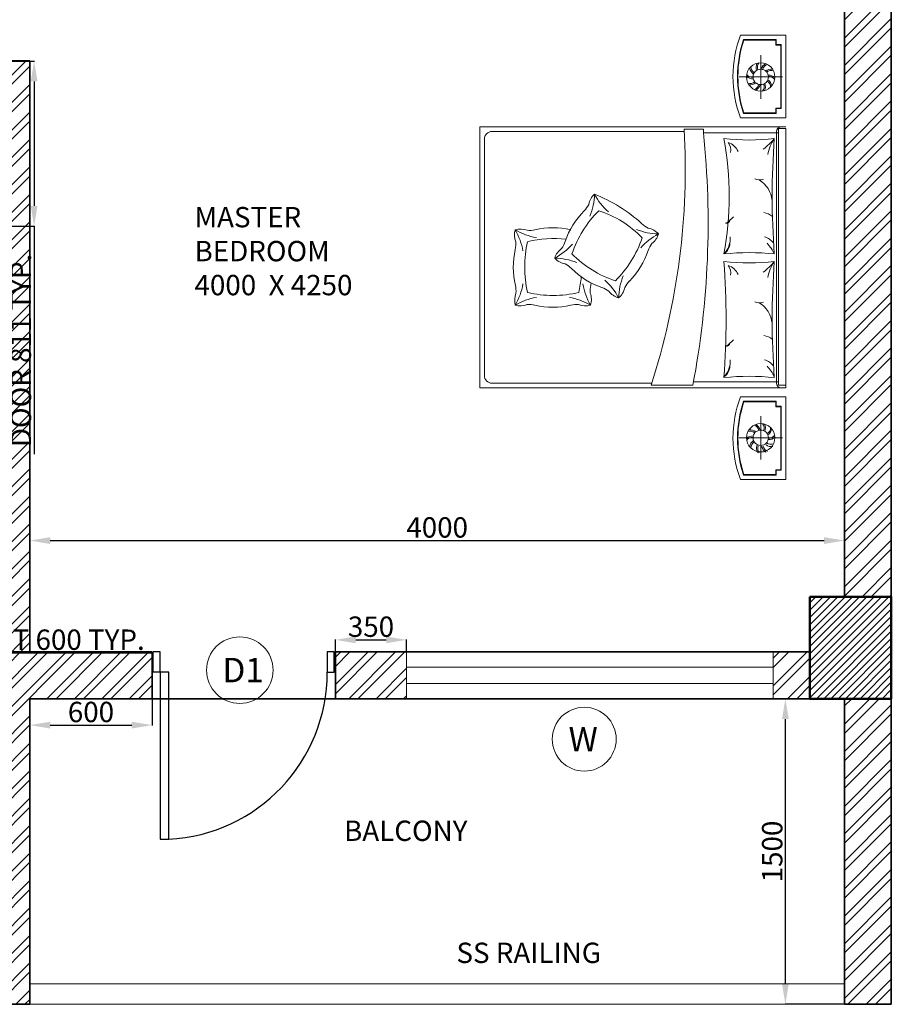
# Model space of a CAD drawing. Units: millimetres. Extents: x -3326 to 29338, y -16792 to 6002.
# Tile 16 of 21: x 25002 to 29282, y -12764 to -7931. Entities that reach past the tile are written whole.
import ezdxf

# ---------------------------------------------------------------- set-up
doc = ezdxf.new("R2010")
doc.units = ezdxf.units.MM
doc.header["$PDMODE"] = 35
doc.header["$PDSIZE"] = 5
for name, color, linetype, lineweight in [('A-ANNO-DIMS', 2, 'Continuous', 13), ('A-ANNO-SYMB', 7, 'Continuous', 18), ('A-AREA-IDEN', 7, 'Continuous', 18), ('A-COLS', 1, 'Continuous', 50), ('A-COLS-PATT', 251, 'Continuous', 13), ('A-DOOR', 3, 'Continuous', 25), ('A-FLOR-RAIL', 8, 'Continuous', 20), ('A-GLAZ', 4, 'Continuous', 18), ('A-WALL', 7, 'Continuous', 35), ('A-WALL-PATT', 252, 'Continuous', 13), ('furn', 28, 'Continuous', 18), ('txt', 7, 'Continuous', 18)]:
    doc.layers.add(name, color=color, linetype=linetype, lineweight=lineweight)
doc.styles.get("Standard").update_dxf_attribs({"font": 'arial.ttf'})
doc.dimstyles.new('ISO-25', dxfattribs={"dimtxt": 100, "dimasz": 100, "dimexe": 1.25, "dimexo": 0.625, "dimtad": 1, "dimtxsty": 'Standard', "dimcen": 2.5, "dimadec": 0, "dimazin": 0, "dimtfac": 1, "dimtmove": 0, "dimatfit": 3, "dimfxl": 1, "dimarcsym": 0})

# ---------------------------------------------------------------- blocks, each defined once
blk = doc.blocks.new('A$C0CE462CD')
for p, q in [((860, 100), (860, 0)), ((860, 0), (893.9, 0))]:
    blk.add_line(p, q)
for points in [[(860, 100), (860, 920), (818.4, 920), (818.4, 100)], [(0, 10), (6.1, 10), (6.1, 90), (0, 90)], [(893.9, 10), (900, 10), (900, 90), (893.9, 90)]]:
    blk.add_lwpolyline(points, close=True)
for points in [[(6.1, 0), (40, 0), (40, 100), (6.1, 100)], [(6.1, 100), (6.1, 0)], [(860, 100), (893.9, 100), (893.9, 0)]]:
    blk.add_lwpolyline(points)
blk.add_arc((859.1, 101.9), 819.1, 92.8508, 180.1309)
blk = doc.blocks.new('*D12')
at = {"layer": 'A-ANNO-DIMS', "color": 0, "lineweight": -2, "transparency": 16777216}
for p, q in [((29051.7, -11264), (28760.9, -11264)), ((28762.1, -12664), (28762.1, -11364)), ((29051.7, -12764), (28760.9, -12764))]:
    blk.add_line(p, q, dxfattribs=at)
at = {"layer": 'A-ANNO-DIMS', "color": 0, "transparency": 16777216}
for points in [[(28745.4, -11364), (28778.8, -11364), (28762.1, -11264)], [(28745.4, -12664), (28778.8, -12664), (28762.1, -12764)]]:
    blk.add_solid(points, dxfattribs=at)
at = {"layer": 'Defpoints', "color": 0, "transparency": 16777216}
for p in [(28762.1, -11264), (29052.3, -11264), (29052.3, -12764)]:
    blk.add_point(p, dxfattribs=at)
at = {"layer": 'A-ANNO-DIMS', "color": 0, "transparency": 16777216, "insert": (28710.4, -12014), "char_height": 100, "attachment_point": 5, "rotation": 90}
blk.add_mtext('1500', dxfattribs=at)
blk = doc.blocks.new('*D13')
at = {"layer": 'A-ANNO-DIMS', "color": 0, "lineweight": -2, "transparency": 16777216}
for p, q in [((25052.3, -11264.6), (25052.3, -11395)), ((25652.3, -11264.6), (25652.3, -11395)), ((25152.3, -11393.8), (25552.3, -11393.8))]:
    blk.add_line(p, q, dxfattribs=at)
at = {"layer": 'A-ANNO-DIMS', "color": 0, "transparency": 16777216}
for points in [[(25152.3, -11377.1), (25152.3, -11410.4), (25052.3, -11393.8)], [(25552.3, -11377.1), (25552.3, -11410.4), (25652.3, -11393.8)]]:
    blk.add_solid(points, dxfattribs=at)
at = {"layer": 'Defpoints', "color": 0, "transparency": 16777216}
for p in [(25052.3, -11264), (25652.3, -11264), (25652.3, -11393.8)]:
    blk.add_point(p, dxfattribs=at)
at = {"layer": 'A-ANNO-DIMS', "color": 0, "transparency": 16777216, "insert": (25352.3, -11342.1), "char_height": 100, "attachment_point": 5}
blk.add_mtext('600', dxfattribs=at)
blk = doc.blocks.new('*D14')
at = {"layer": 'A-ANNO-DIMS', "color": 0, "lineweight": -2, "transparency": 16777216}
for p, q in [((26552.3, -11033.3), (26552.3, -10973.9)), ((26652.3, -10975.2), (26802.3, -10975.2)), ((26902.3, -11033.3), (26902.3, -10973.9))]:
    blk.add_line(p, q, dxfattribs=at)
at = {"layer": 'A-ANNO-DIMS', "color": 0, "transparency": 16777216}
for points in [[(26652.3, -10958.5), (26652.3, -10991.9), (26552.3, -10975.2)], [(26802.3, -10958.5), (26802.3, -10991.9), (26902.3, -10975.2)]]:
    blk.add_solid(points, dxfattribs=at)
at = {"layer": 'Defpoints', "color": 0, "transparency": 16777216}
for p in [(26902.3, -10975.2), (26552.3, -11034), (26902.3, -11034)]:
    blk.add_point(p, dxfattribs=at)
at = {"layer": 'A-ANNO-DIMS', "color": 0, "transparency": 16777216, "insert": (26727.3, -10923.5), "char_height": 100, "attachment_point": 5}
blk.add_mtext('350', dxfattribs=at)
blk = doc.blocks.new('*D15')
at = {"layer": 'A-ANNO-DIMS', "color": 0, "lineweight": -2, "transparency": 16777216}
for p, q in [((29052.3, -10333.7), (29052.3, -10489.2)), ((25052.3, -10425.5), (25052.3, -10489.2)), ((25152.3, -10487.9), (28952.3, -10487.9))]:
    blk.add_line(p, q, dxfattribs=at)
at = {"layer": 'A-ANNO-DIMS', "color": 0, "transparency": 16777216}
for points in [[(25152.3, -10471.3), (25152.3, -10504.6), (25052.3, -10487.9)], [(28952.3, -10471.3), (28952.3, -10504.6), (29052.3, -10487.9)]]:
    blk.add_solid(points, dxfattribs=at)
at = {"layer": 'Defpoints', "color": 0, "transparency": 16777216}
for p in [(29052.3, -10333.1), (25052.3, -10424.9), (29052.3, -10487.9)]:
    blk.add_point(p, dxfattribs=at)
at = {"layer": 'A-ANNO-DIMS', "color": 0, "transparency": 16777216, "insert": (27052.3, -10436.3), "char_height": 100, "attachment_point": 5}
blk.add_mtext('4000', dxfattribs=at)
blk = doc.blocks.new('BED-WITH-NIGHTSTANDS')
for p, q in [((1378.9, 2083.2), (1378.9, 1869.8)), ((1272.3, 1976.5), (1485.6, 1976.5)), ((1466.8, 1702.3), (1097.4, 1702.3)), ((1455.8, 1708.6), (1455.8, 473.4)), ((1466.8, 480.5), (1049.3, 480.5)), ((1378.9, 98.8), (1378.9, 312.2)), ((1272.2, 205.5), (1485.6, 205.5))]:
    blk.add_line(p, q)
for points in [[(1279.5, 2182), (1501.4, 2182), (1501.4, 1775.2), (1279.5, 1775.2, -0.181818)], [(1097.4, 1719.6), (1097.4, 1702.3, -0.072944), (1045.8, 463.1), (840.6, 463.1, 0.092568), (1003.3, 1719.6)], [(1198.4, 1674.1, 0.058596), (1445.6, 1674.1, 0.036889), (1445.6, 1107.7, 0.052163), (1198.4, 1107.7, 0.093111)], [(1198.4, 1070.9, 0.058596), (1445.6, 1070.9, 0.036648), (1445.6, 500.8, 0.052163), (1198.4, 500.8, 0.036967)], [(1279.6, 0), (1501.5, 0), (1501.5, 406.8), (1279.6, 406.8, 0.181818)]]:
    blk.add_lwpolyline(points, format="xyb", close=True)
for points in [[(1454.8, 1797.4), (1295, 1797.4, -0.167087), (1295, 2159.8), (1454.8, 2159.8)], [(1454.8, 1799.6), (1296.6, 1799.6, -0.165559), (1296.6, 2157.6), (1454.8, 2157.6)], [(1003.9, 1708.6), (59.2, 1708.6, 0.414214), (22.2, 1671.6), (22.2, 510.4, 0.414214), (59.2, 473.4), (844.2, 473.4)], [(540, 1293.1, 0.091296), (562.8, 1401.4, 0.091296), (630.7, 1314.1, 0.091296)], [(583.2, 1320, 0.111006), (451.8, 1108.7, 0.119549), (665.6, 975.5, 0.107813), (797.5, 1186.1)], [(797.2, 1187.3, 0.121865), (583.2, 1319.9, 0.121865)], [(211.2, 1122.2, 0.091296), (173.3, 1226.2, 0.091296), (277.2, 1187.9, 0.091296)], [(768.3, 1228.3, 0.091296), (876.7, 1205.8, 0.091296), (789.5, 1137.6, 0.091296)], [(233.7, 1167.8, 0.111006), (234, 919, 0.119549), (485.8, 919, 0.033212), (497.4, 995.5)], [(475.6, 1065.1, 0.091296), (367.2, 1087.5, 0.091296), (454.4, 1155.8)], [(367.2, 1087.5, 0.159461), (418, 1058.9, -0.076283), (449.6, 1036.2, 0.115075), (598.7, 943.3, -0.076283), (633, 924.9, 0.159461), (681.1, 892)], [(703.9, 1000.2, 0.091296), (681.1, 892, 0.091296), (613.2, 979.3, 0.091296)], [(277.2, 894.6, 0.091296), (173.3, 856.3, 0.091296), (211.2, 960.3)], [(505.3, 960.3, 0.091296), (543.2, 856.3, 0.091296), (439.3, 894.6, 0.091296)], [(173.3, 856.3, 0.159461), (231.6, 858.9, -0.076283), (270.5, 856.3, 0.115075), (446, 856.3, -0.076283), (484.9, 858.9, 0.159461), (543.2, 856.3)], [(1454.9, 384.6), (1295.1, 384.6, 0.167087), (1295.1, 22.2), (1454.9, 22.2)], [(1454.9, 382.4), (1296.7, 382.4, 0.165559), (1296.7, 24.4), (1454.9, 24.4)]]:
    blk.add_lwpolyline(points, format="xyb")
for points in [[(1479.2, 2133.2), (1452.6, 2133.2), (1452.6, 2159.8)], [(1479.2, 2135.4), (1454.8, 2135.4), (1454.8, 2159.8)], [(1477, 2135.4), (1477, 1821.8)], [(1479.2, 2135.4), (1479.2, 1821.8)], [(1479.2, 1824), (1452.6, 1824), (1452.6, 1797.4)], [(1479.2, 1821.8), (1454.8, 1821.8), (1454.8, 1797.4)], [(1501.5, 1730.8), (0, 1730.8), (0, 451.2), (1501.5, 451.2)], [(1501.5, 463.1), (1466.8, 463.1), (1466.8, 1723.4), (1501.5, 1723.4), (1501.5, 451.2)], [(1479.3, 358), (1452.7, 358), (1452.7, 384.6)], [(1479.3, 360.2), (1454.9, 360.2), (1454.9, 384.6)], [(1477.1, 46.6), (1477.1, 360.2)], [(1479.3, 46.6), (1479.3, 360.2)], [(1479.3, 48.8), (1452.7, 48.8), (1452.7, 22.2)], [(1479.3, 46.6), (1454.9, 46.6), (1454.9, 22.2)]]:
    blk.add_lwpolyline(points)
for centre, radius in [((1378.9, 1976.5), 69.7), ((1378.9, 1976.5), 37.8), ((1378.9, 205.5), 69.7), ((1378.9, 205.5), 37.8)]:
    blk.add_circle(centre, radius)
for centre, radius, start, end in [((1400.9, 2024.2), 44.8, 154.17, 200.4897), ((1396.5, 2024.6), 34.1, 142.3002, 202.538), ((1424.8, 2002.2), 44.8, 118.17, 164.4897), ((1421.4, 2005.1), 34.1, 106.3002, 166.538), ((1338.5, 2008.1), 34.1, 214.3002, 274.538), ((1368.7, 2028), 44.8, 190.17, 236.4897), ((1364.8, 2025.8), 34.1, 178.3002, 238.538), ((1431.1, 1970.3), 44.8, 82.17, 128.4897), ((1430.1, 1974.7), 34.1, 70.3002, 130.538), ((1417.5, 1940.8), 44.8, 46.17, 92.4897), ((1340.3, 2012.2), 44.8, 226.17, 272.4897), ((1327.7, 1978.3), 34.1, 250.3002, 310.538), ((1326.7, 1982.7), 44.8, 262.17, 308.4897), ((1336.4, 1947.9), 34.1, 286.3002, 346.538), ((1333.1, 1950.8), 44.8, 298.17, 344.4897), ((1361.4, 1928.3), 34.1, 322.3002, 22.538), ((1356.9, 1928.8), 44.8, 334.17, 20.4897), ((1393, 1927.2), 34.1, 358.3002, 58.538), ((1389.2, 1925), 44.8, 10.17, 56.4897), ((1419.3, 1944.9), 34.1, 34.3002, 94.538), ((1478, 1708.6), 22.2, 90, 180), ((1175.6, 1619.4), 56.2, 346.4823, 38.5563), ((1192.7, 1576.7), 82.2, 24.2916, 70.9896), ((1214.5, 1859.4), 296.3, 306.4935, 321.2792), ((1652.3, 1542.6), 244.9, 147.5379, 167.5233), ((1375.3, 1532.7), 61.4, 245.8927, 286.1192), ((1299.1, 1354.7), 137.1, 6.6849, 58.3182), ((626.3, 1332.5), 93.8, 132.6522, 168.8929), ((256.3, 651.7), 810, 48.3818, 67.7644), ((785.6, 1046.2), 386.5, 135.1307, 161.3884), ((419.7, 1408.4), 128.4, 315.7718, 333.2208), ((1377, 1216.1), 96.2, 51.8174, 79.8987), ((884.1, 1348.9), 128.4, 225.5854, 243.0343), ((1208.9, 1279), 20.7, 263.7543, 347.2187), ((1026.5, 1507.4), 308.8, 306.2085, 315.0849), ((263.7, 1201.2), 93.8, 164.5791, 200.8198), ((198.5, 1135.9), 93.8, 69.3666, 105.6073), ((242.7, 1351.6), 128.4, 265.0387, 282.4877), ((358.2, 849.8), 386.5, 76.8711, 103.1289), ((807.5, 1142.5), 93.8, 42.4658, 78.7065), ((48.2, 1156.4), 128.4, 347.6988, 5.1477), ((360.8, 659.2), 524.3, 83.1956, 104.0284), ((298.1, 1211.9), 128.4, 323.2983, 340.7472), ((789.7, 1230.6), 90.5, 307.2937, 344.0973), ((1127.7, 1179.9), 101.1, 314.406, 6.8342), ((1163, 1161), 64, 303.6349, 0.8456), ((1363.4, 1094.5), 103.5, 40.5354, 70.3558), ((550.3, 1042.5), 386.5, 167.0576, 193.3153), ((468.2, 1051.5), 107.3, 128.7754, 160.3571), ((460, 1247.6), 386.5, 315.1307, 341.3884), ((947.4, 1081.9), 128.4, 143.2983, 160.7472), ((1276.2, 1030), 186.4, 24.6457, 44.1585), ((1214.5, 1256.2), 296.3, 306.4935, 321.2792), ((1652.3, 939.4), 244.9, 147.5379, 167.5233), ((1175.6, 1016.2), 56.2, 346.4823, 38.5563), ((1192.7, 973.5), 82.2, 24.2916, 70.9896), ((825.9, 885.4), 128.4, 135.7718, 153.2208), ((48.9, 925.3), 128.4, 355.2252, 12.6741), ((669.5, 927.3), 128.4, 167.6988, 185.1477), ((167.4, 1041.2), 386.5, 347.0576, 348.7033), ((626.1, 958.8), 86.6, 309.4726, 349.6505), ((278.1, 879.2), 107.3, 160.7023, 192.284), ((461.1, 884), 86.6, 341.3996, 21.5774), ((1375.3, 929.5), 61.4, 245.8927, 286.1192), ((1299.1, 751.6), 137.1, 6.6849, 58.3182), ((1026.5, 904.2), 308.8, 306.2085, 315.0849), ((1377, 612.9), 96.2, 51.8174, 79.8987), ((1208.9, 675.8), 20.7, 263.7543, 347.2187), ((1127.7, 576.7), 101.1, 314.406, 6.8342), ((1363.4, 491.3), 103.5, 40.5354, 70.3558), ((1163, 557.8), 64, 303.6349, 0.8456), ((1276.2, 426.8), 186.4, 24.6457, 44.1585), ((1478, 473.4), 22.2, 180, 270), ((1326.7, 199.3), 44.8, 51.5103, 97.83), ((1336.4, 234.2), 34.1, 13.462, 73.6998), ((1333, 231.2), 44.8, 15.5103, 61.83), ((1361.4, 253.7), 34.1, 337.462, 37.6998), ((1356.9, 253.2), 44.8, 339.5103, 25.83), ((1393, 254.8), 34.1, 301.462, 1.6998), ((1389.2, 257.1), 44.8, 303.5103, 349.83), ((1340.3, 169.8), 44.8, 87.5103, 133.83), ((1338.5, 173.9), 34.1, 85.462, 145.6998), ((1327.7, 203.7), 34.1, 49.462, 109.6998), ((1417.5, 241.2), 44.8, 267.5103, 313.83), ((1419.3, 237.1), 34.1, 265.462, 325.6998), ((1368.6, 154), 44.8, 123.5103, 169.83), ((1364.8, 156.2), 34.1, 121.462, 181.6998), ((1402.8, 152.7), 44.8, 159.5103, 205.83), ((1398.4, 152.3), 34.1, 157.462, 217.6998), ((1426.7, 174.7), 44.8, 195.5103, 241.83), ((1423.3, 171.8), 34.1, 193.462, 253.6998), ((1433, 206.6), 44.8, 231.5103, 277.83), ((1430.1, 207.3), 34.1, 229.462, 289.6998)]:
    blk.add_arc(centre, radius, start, end)
blk = doc.blocks.new('TAG-D1')
blk.add_circle((163.3, 163.3), 163.3)
at = {"insert": (78, 223.5), "char_height": 120, "attachment_point": 1}
blk.add_mtext_dynamic_manual_height_columns('D1', width=137.943, gutter_width=12.5, heights=[0], dxfattribs=at)
blk = doc.blocks.new('TAG-W')
blk.add_circle((156.8, 156.8), 156.8)
at = {"insert": (79.7, 216.8), "char_height": 120, "attachment_point": 1}
blk.add_mtext_dynamic_manual_height_columns('W', width=376.575, gutter_width=12.5, heights=[0], dxfattribs=at)
blk = doc.blocks.new('GLAZ-1800x80')
for p, q in [((0, 80), (1800, 80)), ((0, 0), (1800, 0))]:
    blk.add_line(p, q)
blk = doc.blocks.new('*D189')
at = {"layer": 'A-ANNO-DIMS', "color": 0, "lineweight": -2, "transparency": 16777216}
for p, q in [((24952.2, -8134.2), (25074.5, -8134.2)), ((25073.2, -8234.2), (25073.2, -8845.3)), ((24952.2, -8945.3), (25074.5, -8945.3)), ((25073.2, -8945.3), (25073.2, -10063.9))]:
    blk.add_line(p, q, dxfattribs=at)
at = {"layer": 'A-ANNO-DIMS', "color": 0, "transparency": 16777216}
for points in [[(25056.6, -8234.2), (25089.9, -8234.2), (25073.2, -8134.2)], [(25056.6, -8845.3), (25089.9, -8845.3), (25073.2, -8945.3)]]:
    blk.add_solid(points, dxfattribs=at)
at = {"layer": 'Defpoints', "color": 0, "transparency": 16777216}
for p in [(24951.6, -8134.2), (24951.6, -8945.3), (25073.2, -8945.3)]:
    blk.add_point(p, dxfattribs=at)
at = {"layer": 'A-ANNO-DIMS', "color": 0, "transparency": 16777216, "insert": (25020.9, -9554.6), "char_height": 100, "attachment_point": 5, "rotation": 90}
blk.add_mtext('DOOR 811 TYP.', dxfattribs=at)
blk = doc.blocks.new('*D205')
at = {"layer": 'A-ANNO-DIMS', "color": 0, "lineweight": -2, "transparency": 16777216}
for p, q in [((23972.3, -11128.3), (23972.3, -11037.7)), ((24072.3, -11039), (24472.3, -11039)), ((24572.3, -11128.3), (24572.3, -11037.7)), ((24572.3, -11039), (25654.6, -11039))]:
    blk.add_line(p, q, dxfattribs=at)
at = {"layer": 'A-ANNO-DIMS', "color": 0, "transparency": 16777216}
for points in [[(24072.3, -11022.3), (24072.3, -11055.6), (23972.3, -11039)], [(24472.3, -11022.3), (24472.3, -11055.6), (24572.3, -11039)]]:
    blk.add_solid(points, dxfattribs=at)
at = {"layer": 'Defpoints', "color": 0, "transparency": 16777216}
for p in [(24572.3, -11039), (23972.3, -11129), (24572.3, -11129)]:
    blk.add_point(p, dxfattribs=at)
at = {"layer": 'A-ANNO-DIMS', "color": 0, "transparency": 16777216, "insert": (25163.4, -10987.3), "char_height": 100, "attachment_point": 5}
blk.add_mtext('VENT 600 TYP.', dxfattribs=at)

msp = doc.modelspace()

# ---------------------------------------------------------------- hatches: boundary and pattern name
at = {"layer": 'A-COLS-PATT'}
h = msp.add_hatch(dxfattribs=at)
h.set_pattern_fill('ANSI31', color=256, scale=8)
h.set_pattern_definition([(45, (-15733.41, -5550.314), (-17.960512, 17.960512), [])])
h.paths.add_polyline_path([(28882.301, -10763.952), (28882.301, -11263.952), (29282.301, -11263.952), (29282.301, -10763.952)])
at = {"layer": 'A-WALL-PATT'}
h = msp.add_hatch(dxfattribs=at)
h.set_pattern_fill('ANSI32', color=256, scale=10)
h.set_pattern_definition([(45, (-10476.65, 1e-12), (-67.35192, 67.35192), []), (45, (-10431.74, 1e-12), (-67.35192, 67.35192), [])])
h.paths.add_polyline_path([(29282.301, -7283.952), (28882.301, -7283.952), (28882.301, -7383.952), (29052.301, -7383.952), (29052.301, -10763.952), (29282.301, -10763.952)])
h.paths.add_polyline_path([(29282.301, -11263.952), (29052.301, -11263.952), (29052.301, -12763.952), (29282.301, -12763.952)])
h.paths.add_polyline_path([(25052.301, -11263.952), (25652.301, -11263.952), (25652.301, -11123.904), (25652.289, -11123.904), (25652.289, -11033.952), (25052.301, -11033.952), (24572.301, -11033.952), (24572.301, -11263.952), (24822.301, -11263.952), (24822.301, -12763.952), (25052.301, -12763.952)])
h.paths.add_polyline_path([(26902.301, -11033.952), (26552.301, -11033.952), (26552.301, -11263.952), (26902.301, -11263.952)])
h.paths.add_polyline_path([(21992.301, -6683.952), (21362.301, -6683.952), (17512.301, -6683.952), (17512.301, -6783.952), (21362.301, -6783.952), (21992.301, -6783.952)])
h.paths.add_polyline_path([(17512.301, -7283.952), (17282.301, -7283.952), (17282.301, -12163.952), (17512.301, -12163.952), (17512.301, -11263.952), (18112.301, -11263.952), (18112.301, -11033.952), (17512.301, -11033.952)])
h.paths.add_polyline_path([(21462.301, -8211.864), (21462.064, -8211.864), (21462.064, -8142.609), (21462.301, -8133.952), (21362.301, -8133.952), (21362.301, -8233.952), (21362.301, -11033.952), (21162.301, -11033.952), (21162.301, -11263.952), (21362.301, -11263.952), (21362.301, -12763.952), (21592.301, -12763.952), (21592.301, -11263.952), (21992.301, -11263.952), (21992.301, -11033.952), (21592.301, -11033.952), (21462.301, -11033.952)])
h.paths.add_polyline_path([(24152.301, -8133.952), (23322.301, -8133.952), (23322.301, -7433.952), (23092.301, -7433.952), (23092.301, -8133.952), (22241.021, -8133.952), (22241.021, -8142.609), (22241.182, -8142.609), (22241.182, -8211.864), (22241.021, -8233.952), (23092.301, -8233.952), (23092.301, -10513.206), (23322.301, -10513.206), (23322.301, -8233.952), (24152.301, -8233.952)])
h.paths.add_polyline_path([(25052.301, -8233.952), (25052.301, -8133.952), (24952.301, -8133.952), (24952.301, -11033.952), (25052.301, -11033.952)])
h.paths.add_polyline_path([(23972.301, -11033.952), (23493.251, -11033.952), (23493.251, -11263.952), (23972.301, -11263.952)])
h.paths.add_polyline_path([(23092.301, -11033.952), (22592.301, -11033.952), (22592.301, -11263.952), (23092.301, -11263.952)])
h.paths.add_polyline_path([(28882.301, -11033.952), (28702.301, -11033.952), (28702.301, -11263.952), (28882.301, -11263.952)])
h.paths.add_polyline_path([(17512.301, -3883.952), (17387.589, -3883.952), (17387.589, -3888.07), (17282.301, -3888.07), (17282.301, -6683.952), (17512.301, -6683.952)])
h.paths.add_polyline_path([(21462.301, -2183.952), (21362.301, -2183.952), (21362.301, -2383.952), (17282.301, -2383.952), (17282.301, -2483.952), (17512.301, -2483.952), (21462.301, -2483.952)])
h.paths.add_polyline_path([(17512.301, -2483.952), (17282.301, -2483.952), (17282.301, -2833.952), (17512.301, -2833.952)])
h.paths.add_polyline_path([(21462.301, 1866.048), (21992.301, 1866.048), (21992.301, 2096.048), (21592.301, 2096.048), (21592.301, 3596.048), (21362.301, 3596.048), (21362.301, 1866.048), (21362.301, -1283.952), (21462.301, -1283.952)])
h.paths.add_polyline_path([(17512.301, 1496.048), (17282.301, 1496.048), (17282.301, -1983.952), (17612.301, -1983.952), (17612.301, -1883.952), (17512.301, -1883.952)])
h.paths.add_polyline_path([(17512.301, 3596.048), (17282.301, 3596.048), (17282.301, 2096.048), (17512.301, 2096.048)])
h.paths.add_polyline_path([(18135.023, 2096.048), (17685.023, 2096.048), (17685.023, 1866.048), (18135.023, 1866.048), (18135.023, 1876.048), (18128.942, 1876.048), (18128.942, 1956.048), (18135.023, 1956.048)])
h.paths.add_polyline_path([(19385.023, 2096.048), (19035.023, 2096.048), (19035.023, 1866.048), (19385.023, 1866.048)])
h.paths.add_polyline_path([(21362.301, 2096.048), (21185.023, 2096.048), (21185.023, 1866.048), (21362.301, 1866.048)])
h.paths.add_polyline_path([(23092.301, 2096.048), (22592.301, 2096.048), (22592.301, 1866.048), (23092.301, 1866.048)])
h.paths.add_polyline_path([(23972.301, 2096.048), (23492.301, 2096.048), (23492.301, 1866.048), (23972.301, 1866.048)])
h.paths.add_polyline_path([(23972.301, 2496.048), (23872.301, 2496.048), (23872.301, 2096.048), (23972.301, 2096.048)])
h.paths.add_polyline_path([(22692.301, 2496.048), (22592.301, 2496.048), (22592.301, 2096.048), (22692.301, 2096.048)])
h.paths.add_polyline_path([(23322.301, 1346.048), (23092.301, 1346.048), (23092.301, -1733.952), (23322.301, -1733.952)])
h.paths.add_polyline_path([(23092.301, -933.952), (22262.301, -933.952), (22262.301, -1033.952), (23092.301, -1033.952)])
h.paths.add_polyline_path([(24952.301, -1433.952), (24952.301, -1733.952), (23492.301, -1733.952), (23492.301, -1833.952), (24952.301, -1833.952), (24952.301, -2483.952), (25052.301, -2483.952), (25052.301, -2466.23), (25049.26, -2466.23), (25049.26, -2386.23), (25049.941, -1433.952)])
h.paths.add_polyline_path([(22692.301, -11263.952), (22592.301, -11263.952), (22592.301, -11663.952), (22692.301, -11663.952)])
h.paths.add_polyline_path([(23972.301, -11263.952), (23872.301, -11263.952), (23872.301, -11663.952), (23972.301, -11663.952)])

# ---------------------------------------------------------------- linework, layer by layer
at = {"layer": 'A-COLS'}
msp.add_lwpolyline([(28882.301, -10763.952), (29282.301, -10763.952), (29282.301, -11263.952), (28882.301, -11263.952)], close=True, dxfattribs=at)
at = {"layer": 'A-FLOR-RAIL'}
for p, q in [((29052.301, -12663.952), (25052.301, -12663.952)), ((29052.301, -12763.952), (25052.301, -12763.952))]:
    msp.add_line(p, q, dxfattribs=at)
at = {"layer": 'A-GLAZ'}
for p, q in [((26902.301, -11033.952), (26902.301, -11263.952)), ((28702.301, -11033.952), (28702.301, -11263.952))]:
    msp.add_line(p, q, dxfattribs=at)
at = {"layer": 'A-WALL'}
for p, q in [((29282.301, -6683.952), (29282.301, -12763.952)), ((29052.301, -7383.952), (29052.301, -10763.952)), ((25052.301, -8133.952), (23322.301, -8133.952)), ((25052.301, -8133.952), (25052.301, -8233.952)), ((25052.301, -8233.952), (25052.301, -11033.952)), ((25052.301, -11033.952), (23493.251, -11033.952)), ((25652.301, -11033.952), (25052.301, -11033.952)), ((25652.301, -11033.952), (25652.301, -11263.952)), ((26552.301, -11033.952), (26552.301, -11263.952)), ((28882.301, -11033.952), (26552.301, -11033.952)), ((29052.301, -11263.952), (25052.301, -11263.952)), ((25052.301, -11263.952), (25052.301, -12763.952)), ((29052.301, -11263.952), (29052.301, -12763.952)), ((25052.301, -12763.952), (24822.301, -12763.952)), ((29282.301, -12763.952), (29052.301, -12763.952))]:
    msp.add_line(p, q, dxfattribs=at)

# ---------------------------------------------------------------- block references
at = {"layer": 'A-ANNO-SYMB'}
for name, p in [('TAG-D1', (25919.85, -11287.022)), ('TAG-W', (27617.645, -11619.541))]:
    msp.add_blockref(name, p, dxfattribs=at)
at = {"layer": 'A-DOOR', "rotation": 180}
msp.add_blockref('A$C0CE462CD', (26552.289, -11033.904), dxfattribs=at)
at = {"layer": 'A-GLAZ'}
msp.add_blockref('GLAZ-1800x80', (26902.301, -11188.952), dxfattribs=at)
at = {"layer": 'furn'}
msp.add_blockref('BED-WITH-NIGHTSTANDS', (27262.132, -10188.793), dxfattribs=at)

# ---------------------------------------------------------------- texts
at = {"layer": 'A-AREA-IDEN', "char_height": 100, "attachment_point": 1}
for s, insert in [('MASTER\\PBEDROOM\\P4000  X 4250', (25860.777, -8850.433)), ('BALCONY', (26595.138, -11862.223))]:
    msp.add_mtext_dynamic_manual_height_columns(s, width=1168.90663, gutter_width=12.5, heights=[0], dxfattribs=dict(at, insert=insert))
at = {"layer": 'txt', "insert": (27146.953, -12461.305), "char_height": 100, "attachment_point": 1}
msp.add_mtext_dynamic_manual_height_columns('SS RAILING', width=1168.90663, gutter_width=12.5, heights=[0], dxfattribs=at)

# ---------------------------------------------------------------- dimensions: what is measured, and where the dimension line sits
at = {"layer": 'A-ANNO-DIMS'}
dim = msp.add_linear_dim(base=(25073.237, -8945.279), p1=(24951.581, -8134.238), p2=(24951.581, -8945.279), angle=270, text='DOOR <> TYP.', dimstyle='ISO-25', override={"dimdec": 0, "dimlfac": 1, "dimrnd": 0, "dimzin": 0, "dimdsep": 46, "dimlunit": 2}, dxfattribs=at)
dim.commit()
dim.dimension.update_dxf_attribs({"geometry": '*D189', "text_midpoint": (25020.872, -9554.601)})
for base, p1, p2, picture, middle in [((29052.301, -10487.944), (25052.301, -10424.856), (29052.301, -10333.093), '*D15', (27052.301, -10436.262)), ((26902.301, -10975.194), (26552.301, -11033.952), (26902.301, -11033.952), '*D14', (26727.301, -10923.478)), ((25652.301, -11393.779), (25052.301, -11263.952), (25652.301, -11263.952), '*D13', (25352.301, -11342.097))]:
    dim = msp.add_linear_dim(base=base, p1=p1, p2=p2, dimstyle='ISO-25', override={"dimclrd": 0, "dimclre": 0, "dimclrt": 0}, dxfattribs=at)
    dim.commit()
    dim.dimension.update_dxf_attribs({"geometry": picture, "text_midpoint": middle})
dim = msp.add_linear_dim(base=(24572.301, -11038.952), p1=(23972.301, -11128.952), p2=(24572.301, -11128.952), text='VENT <> TYP.', dimstyle='ISO-25', override={"dimdec": 0, "dimlfac": 1, "dimrnd": 0, "dimzin": 0, "dimdsep": 46, "dimlunit": 2}, dxfattribs=at)
dim.commit()
dim.dimension.update_dxf_attribs({"geometry": '*D205', "text_midpoint": (25163.444, -10987.27)})
dim = msp.add_linear_dim(base=(28762.11, -11263.952), p1=(29052.301, -12763.952), p2=(29052.301, -11263.952), angle=90, dimstyle='ISO-25', override={"dimclrd": 0, "dimclre": 0, "dimclrt": 0}, dxfattribs=at)
dim.commit()
dim.dimension.update_dxf_attribs({"geometry": '*D12', "text_midpoint": (28710.428, -12013.952)})

doc.saveas('drawing.dxf')
